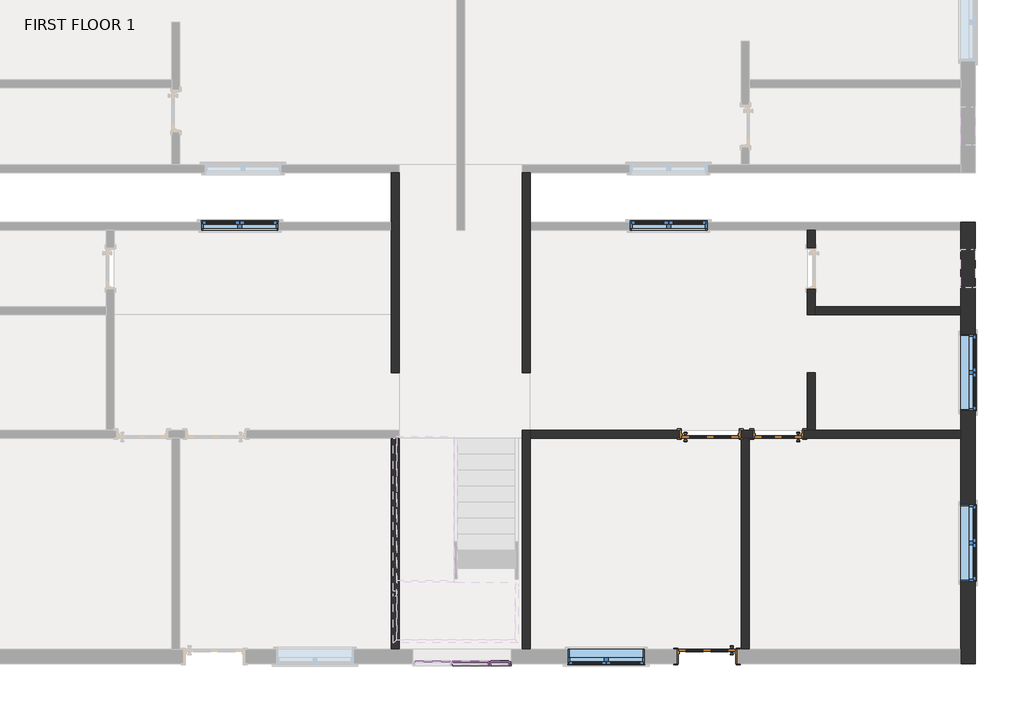
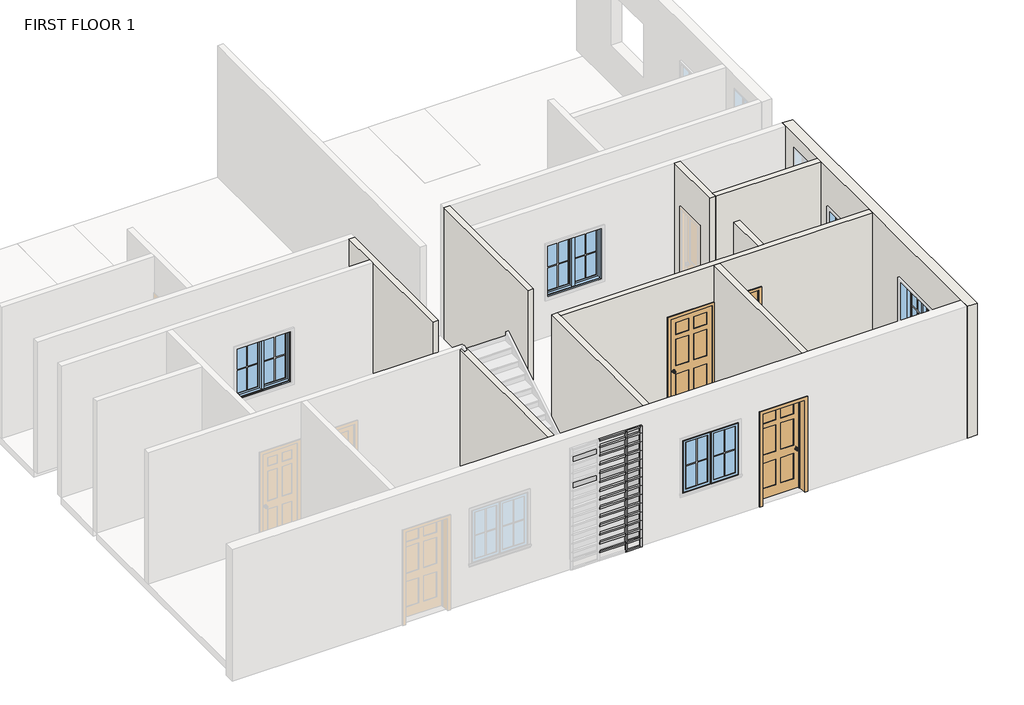
# One storey, part 2 of 4: 57 members, 18 plates, 10 walls, 5 windows, 3 doors.
"""IFC4 building model written with IfcOpenShell, lengths in millimetres."""

from ifc_helpers import new_model, si_unit, frame, origin, place, context, project, spatial, polyline, outline, extrude, faceted_brep, transform, mapped, element, save
from components import door_d66ee888, door_c610b25b, door_c5239341, member_56b223d9, member_a59c64b1, member_06854975, member_b8e7570c, member_a67f877f, member_00eacae2, member_ff422208, member_dc11c383, system_panel_glazed_b3845325, system_panel_glazed_23b8b45c, system_panel_glazed_58d257f9, system_panel_glazed_e426d894, system_panel_glazed_822b3193, window_9200f5ac, window_c2c97eee

model = new_model("IFC4")

# Units and contexts
model_context = context("Model", 3, world=origin())
ifc_project = project(units=[si_unit("LENGTHUNIT", "METRE", prefix="MILLI")], contexts=[model_context])

# Site, building, storey
site = spatial("IfcSite", under=ifc_project)
building = spatial("IfcBuilding", under=site)
storey = spatial("IfcBuildingStorey", under=building, Name="FIRST FLOOR 1", Elevation=3200.4)

# Doors
placement = place(None, origin())
door_shape = door_d66ee888(model_context)
element("IfcDoor", 1, ObjectType="Door-Interior-Single-6_Panel-Wood : 30\" x 84\"", at=placement, inside=storey, context=model_context, shape_type="MappedRepresentation", body=[
    mapped(door_shape, transform((777.5862669, -4180.7343836, 3200.4), x_axis=(-1.0, 0.0, 0.0), y_axis=(0.0, -1.0, 0.0), z_axis=(0.0, 0.0, 1.0))),
])
door_2_shape = door_c610b25b(model_context)
element("IfcDoor", 2, ObjectType="Door-Interior-Single-6_Panel-Wood : 36\" x 84\"", at=placement, inside=storey, context=model_context, shape_type="MappedRepresentation", body=[
    mapped(door_2_shape, transform((-301.9137331, -4180.7343836, 3200.4), x_axis=(1.0, 0.0, 0.0), y_axis=(0.0, 1.0, 0.0), z_axis=(0.0, 0.0, 1.0))),
])
door_3_shape = door_c5239341(model_context)
element("IfcDoor", 3, ObjectType="Door-Interior-Single-6_Panel-Wood : 36\" x 84\"", at=placement, inside=storey, context=model_context, shape_type="MappedRepresentation", body=[
    mapped(door_3_shape, transform((-352.7137331, -7704.9843836, 3200.4), x_axis=(-1.0, 0.0, 0.0), y_axis=(0.0, -1.0, 0.0), z_axis=(0.0, 0.0, 1.0))),
])

# Members
member_shape = member_56b223d9(model_context)
element("IfcMember", 4, ObjectType="Rectangular Mullion : 1.5\" x 2.5\" rectangular", at=placement, inside=storey, context=model_context, shape_type="MappedRepresentation", body=[
    mapped(member_shape, transform((-3807.0334597, -7822.4593836, 3200.4), x_axis=(1.0, 0.0, 0.0), y_axis=(0.0, -1.0, 0.0), z_axis=(0.0, 0.0, -1.0))),
])
element("IfcMember", 5, ObjectType="Rectangular Mullion : 1.5\" x 2.5\" rectangular", at=placement, inside=storey, context=model_context, shape_type="MappedRepresentation", body=[
    mapped(member_shape, transform((-3807.0334597, -7822.4593836, 3403.6), x_axis=(1.0, 0.0, 0.0), y_axis=(0.0, -1.0, 0.0), z_axis=(0.0, 0.0, -1.0))),
])
element("IfcMember", 6, ObjectType="Rectangular Mullion : 1.5\" x 2.5\" rectangular", at=placement, inside=storey, context=model_context, shape_type="MappedRepresentation", body=[
    mapped(member_shape, transform((-3807.0334597, -7822.4593836, 3606.8), x_axis=(1.0, 0.0, 0.0), y_axis=(0.0, -1.0, 0.0), z_axis=(0.0, 0.0, -1.0))),
])
element("IfcMember", 7, ObjectType="Rectangular Mullion : 1.5\" x 2.5\" rectangular", at=placement, inside=storey, context=model_context, shape_type="MappedRepresentation", body=[
    mapped(member_shape, transform((-3807.0334597, -7822.4593836, 3810.0), x_axis=(1.0, 0.0, 0.0), y_axis=(0.0, -1.0, 0.0), z_axis=(0.0, 0.0, -1.0))),
])
element("IfcMember", 8, ObjectType="Rectangular Mullion : 1.5\" x 2.5\" rectangular", at=placement, inside=storey, context=model_context, shape_type="MappedRepresentation", body=[
    mapped(member_shape, transform((-3807.0334597, -7822.4593836, 4013.2), x_axis=(1.0, 0.0, 0.0), y_axis=(0.0, -1.0, 0.0), z_axis=(0.0, 0.0, -1.0))),
])
element("IfcMember", 9, ObjectType="Rectangular Mullion : 1.5\" x 2.5\" rectangular", at=placement, inside=storey, context=model_context, shape_type="MappedRepresentation", body=[
    mapped(member_shape, transform((-3807.0334597, -7822.4593836, 4216.4), x_axis=(1.0, 0.0, 0.0), y_axis=(0.0, -1.0, 0.0), z_axis=(0.0, 0.0, -1.0))),
])
element("IfcMember", 10, ObjectType="Rectangular Mullion : 1.5\" x 2.5\" rectangular", at=placement, inside=storey, context=model_context, shape_type="MappedRepresentation", body=[
    mapped(member_shape, transform((-3807.0334597, -7822.4593836, 4419.6), x_axis=(1.0, 0.0, 0.0), y_axis=(0.0, -1.0, 0.0), z_axis=(0.0, 0.0, -1.0))),
])
element("IfcMember", 11, ObjectType="Rectangular Mullion : 1.5\" x 2.5\" rectangular", at=placement, inside=storey, context=model_context, shape_type="MappedRepresentation", body=[
    mapped(member_shape, transform((-3807.0334597, -7822.4593836, 4622.8), x_axis=(1.0, 0.0, 0.0), y_axis=(0.0, -1.0, 0.0), z_axis=(0.0, 0.0, -1.0))),
])
element("IfcMember", 12, ObjectType="Rectangular Mullion : 1.5\" x 2.5\" rectangular", at=placement, inside=storey, context=model_context, shape_type="MappedRepresentation", body=[
    mapped(member_shape, transform((-3807.0334597, -7822.4593836, 4826.0), x_axis=(1.0, 0.0, 0.0), y_axis=(0.0, -1.0, 0.0), z_axis=(0.0, 0.0, -1.0))),
])
element("IfcMember", 13, ObjectType="Rectangular Mullion : 1.5\" x 2.5\" rectangular", at=placement, inside=storey, context=model_context, shape_type="MappedRepresentation", body=[
    mapped(member_shape, transform((-3807.0334597, -7822.4593836, 5029.2), x_axis=(1.0, 0.0, 0.0), y_axis=(0.0, -1.0, 0.0), z_axis=(0.0, 0.0, -1.0))),
])
element("IfcMember", 14, ObjectType="Rectangular Mullion : 1.5\" x 2.5\" rectangular", at=placement, inside=storey, context=model_context, shape_type="MappedRepresentation", body=[
    mapped(member_shape, transform((-3807.0334597, -7822.4593836, 5232.4), x_axis=(1.0, 0.0, 0.0), y_axis=(0.0, -1.0, 0.0), z_axis=(0.0, 0.0, -1.0))),
])
element("IfcMember", 15, ObjectType="Rectangular Mullion : 1.5\" x 2.5\" rectangular", at=placement, inside=storey, context=model_context, shape_type="MappedRepresentation", body=[
    mapped(member_shape, transform((-3807.0334597, -7822.4593836, 5435.6), x_axis=(1.0, 0.0, 0.0), y_axis=(0.0, -1.0, 0.0), z_axis=(0.0, 0.0, -1.0))),
])
element("IfcMember", 16, ObjectType="Rectangular Mullion : 1.5\" x 2.5\" rectangular", at=placement, inside=storey, context=model_context, shape_type="MappedRepresentation", body=[
    mapped(member_shape, transform((-3807.0334597, -7822.4593836, 5638.8), x_axis=(1.0, 0.0, 0.0), y_axis=(0.0, -1.0, 0.0), z_axis=(0.0, 0.0, -1.0))),
])
member_2_shape = member_a59c64b1(model_context)
element("IfcMember", 17, ObjectType="Rectangular Mullion : 1.5\" x 2.5\" rectangular", at=placement, inside=storey, context=model_context, shape_type="MappedRepresentation", body=[
    mapped(member_2_shape, transform((-3807.0334597, -7822.4593836, 5842.0), x_axis=(1.0, 0.0, 0.0), y_axis=(0.0, -1.0, 0.0), z_axis=(0.0, 0.0, -1.0))),
])
member_3_shape = member_06854975(model_context)
element("IfcMember", 18, ObjectType="Rectangular Mullion : 1.5\" x 2.5\" rectangular", at=placement, inside=storey, context=model_context, shape_type="MappedRepresentation", body=[
    mapped(member_3_shape, transform((-3499.7513929, -7822.4593836, 6007.7826151), x_axis=(0.0, 0.0, 1.0), y_axis=(0.0, -1.0, 0.0), z_axis=(1.0, 0.0, 0.0))),
])
member_4_shape = member_b8e7570c(model_context)
element("IfcMember", 19, ObjectType="Rectangular Mullion : 1.5\" x 2.5\" rectangular", at=placement, inside=storey, context=model_context, shape_type="MappedRepresentation", body=[
    mapped(member_4_shape, transform((-3826.0834597, -7822.4593836, 3403.6), x_axis=(0.0, 0.0, 1.0), y_axis=(0.0, -1.0, 0.0), z_axis=(1.0, 0.0, 0.0))),
])
element("IfcMember", 20, ObjectType="Rectangular Mullion : 1.5\" x 2.5\" rectangular", at=placement, inside=storey, context=model_context, shape_type="MappedRepresentation", body=[
    mapped(member_4_shape, transform((-3826.0834597, -7822.4593836, 3606.8), x_axis=(0.0, 0.0, 1.0), y_axis=(0.0, -1.0, 0.0), z_axis=(1.0, 0.0, 0.0))),
])
element("IfcMember", 21, ObjectType="Rectangular Mullion : 1.5\" x 2.5\" rectangular", at=placement, inside=storey, context=model_context, shape_type="MappedRepresentation", body=[
    mapped(member_4_shape, transform((-3826.0834597, -7822.4593836, 3810.0), x_axis=(0.0, 0.0, 1.0), y_axis=(0.0, -1.0, 0.0), z_axis=(1.0, 0.0, 0.0))),
])
element("IfcMember", 22, ObjectType="Rectangular Mullion : 1.5\" x 2.5\" rectangular", at=placement, inside=storey, context=model_context, shape_type="MappedRepresentation", body=[
    mapped(member_4_shape, transform((-3826.0834597, -7822.4593836, 4013.2), x_axis=(0.0, 0.0, 1.0), y_axis=(0.0, -1.0, 0.0), z_axis=(1.0, 0.0, 0.0))),
])
element("IfcMember", 23, ObjectType="Rectangular Mullion : 1.5\" x 2.5\" rectangular", at=placement, inside=storey, context=model_context, shape_type="MappedRepresentation", body=[
    mapped(member_4_shape, transform((-3826.0834597, -7822.4593836, 4216.4), x_axis=(0.0, 0.0, 1.0), y_axis=(0.0, -1.0, 0.0), z_axis=(1.0, 0.0, 0.0))),
])
element("IfcMember", 24, ObjectType="Rectangular Mullion : 1.5\" x 2.5\" rectangular", at=placement, inside=storey, context=model_context, shape_type="MappedRepresentation", body=[
    mapped(member_4_shape, transform((-3826.0834597, -7822.4593836, 4419.6), x_axis=(0.0, 0.0, 1.0), y_axis=(0.0, -1.0, 0.0), z_axis=(1.0, 0.0, 0.0))),
])
element("IfcMember", 25, ObjectType="Rectangular Mullion : 1.5\" x 2.5\" rectangular", at=placement, inside=storey, context=model_context, shape_type="MappedRepresentation", body=[
    mapped(member_4_shape, transform((-3826.0834597, -7822.4593836, 4622.8), x_axis=(0.0, 0.0, 1.0), y_axis=(0.0, -1.0, 0.0), z_axis=(1.0, 0.0, 0.0))),
])
element("IfcMember", 26, ObjectType="Rectangular Mullion : 1.5\" x 2.5\" rectangular", at=placement, inside=storey, context=model_context, shape_type="MappedRepresentation", body=[
    mapped(member_4_shape, transform((-3826.0834597, -7822.4593836, 4826.0), x_axis=(0.0, 0.0, 1.0), y_axis=(0.0, -1.0, 0.0), z_axis=(1.0, 0.0, 0.0))),
])
element("IfcMember", 27, ObjectType="Rectangular Mullion : 1.5\" x 2.5\" rectangular", at=placement, inside=storey, context=model_context, shape_type="MappedRepresentation", body=[
    mapped(member_4_shape, transform((-3826.0834597, -7822.4593836, 5029.2), x_axis=(0.0, 0.0, 1.0), y_axis=(0.0, -1.0, 0.0), z_axis=(1.0, 0.0, 0.0))),
])
element("IfcMember", 28, ObjectType="Rectangular Mullion : 1.5\" x 2.5\" rectangular", at=placement, inside=storey, context=model_context, shape_type="MappedRepresentation", body=[
    mapped(member_4_shape, transform((-3826.0834597, -7822.4593836, 5232.4), x_axis=(0.0, 0.0, 1.0), y_axis=(0.0, -1.0, 0.0), z_axis=(1.0, 0.0, 0.0))),
])
element("IfcMember", 29, ObjectType="Rectangular Mullion : 1.5\" x 2.5\" rectangular", at=placement, inside=storey, context=model_context, shape_type="MappedRepresentation", body=[
    mapped(member_4_shape, transform((-3826.0834597, -7822.4593836, 5435.6), x_axis=(0.0, 0.0, 1.0), y_axis=(0.0, -1.0, 0.0), z_axis=(1.0, 0.0, 0.0))),
])
element("IfcMember", 30, ObjectType="Rectangular Mullion : 1.5\" x 2.5\" rectangular", at=placement, inside=storey, context=model_context, shape_type="MappedRepresentation", body=[
    mapped(member_4_shape, transform((-3826.0834597, -7822.4593836, 5638.8), x_axis=(0.0, 0.0, 1.0), y_axis=(0.0, -1.0, 0.0), z_axis=(1.0, 0.0, 0.0))),
])
element("IfcMember", 31, ObjectType="Rectangular Mullion : 1.5\" x 2.5\" rectangular", at=placement, inside=storey, context=model_context, shape_type="MappedRepresentation", body=[
    mapped(member_4_shape, transform((-3826.0834597, -7822.4593836, 5842.0), x_axis=(0.0, 0.0, 1.0), y_axis=(0.0, -1.0, 0.0), z_axis=(1.0, 0.0, 0.0))),
])
member_5_shape = member_a67f877f(model_context)
element("IfcMember", 32, ObjectType="Rectangular Mullion : 1.5\" x 2.5\" rectangular", at=placement, inside=storey, context=model_context, shape_type="MappedRepresentation", body=[
    mapped(member_5_shape, transform((-3826.0834597, -7822.4593836, 6007.7826151), x_axis=(0.0, 0.0, 1.0), y_axis=(0.0, -1.0, 0.0), z_axis=(1.0, 0.0, 0.0))),
])
element("IfcMember", 33, ObjectType="Rectangular Mullion : 1.5\" x 2.5\" rectangular", at=placement, inside=storey, context=model_context, shape_type="MappedRepresentation", body=[
    mapped(member_3_shape, transform((-3787.9834597, -7822.4593836, 3200.4), x_axis=(0.0, 0.0, -1.0), y_axis=(0.0, -1.0, 0.0), z_axis=(-1.0, 0.0, 0.0))),
])
member_6_shape = member_00eacae2(model_context)
element("IfcMember", 34, ObjectType="Rectangular Mullion : 1.5\" x 2.5\" rectangular", at=placement, inside=storey, context=model_context, shape_type="MappedRepresentation", body=[
    mapped(member_6_shape, transform((-3499.7513929, -7822.4593836, 3403.6), x_axis=(0.0, 0.0, 1.0), y_axis=(0.0, -1.0, 0.0), z_axis=(1.0, 0.0, 0.0))),
])
element("IfcMember", 35, ObjectType="Rectangular Mullion : 1.5\" x 2.5\" rectangular", at=placement, inside=storey, context=model_context, shape_type="MappedRepresentation", body=[
    mapped(member_6_shape, transform((-3499.7513929, -7822.4593836, 3606.8), x_axis=(0.0, 0.0, 1.0), y_axis=(0.0, -1.0, 0.0), z_axis=(1.0, 0.0, 0.0))),
])
element("IfcMember", 36, ObjectType="Rectangular Mullion : 1.5\" x 2.5\" rectangular", at=placement, inside=storey, context=model_context, shape_type="MappedRepresentation", body=[
    mapped(member_6_shape, transform((-3499.7513929, -7822.4593836, 3810.0), x_axis=(0.0, 0.0, 1.0), y_axis=(0.0, -1.0, 0.0), z_axis=(1.0, 0.0, 0.0))),
])
element("IfcMember", 37, ObjectType="Rectangular Mullion : 1.5\" x 2.5\" rectangular", at=placement, inside=storey, context=model_context, shape_type="MappedRepresentation", body=[
    mapped(member_6_shape, transform((-3499.7513929, -7822.4593836, 4013.2), x_axis=(0.0, 0.0, 1.0), y_axis=(0.0, -1.0, 0.0), z_axis=(1.0, 0.0, 0.0))),
])
element("IfcMember", 38, ObjectType="Rectangular Mullion : 1.5\" x 2.5\" rectangular", at=placement, inside=storey, context=model_context, shape_type="MappedRepresentation", body=[
    mapped(member_6_shape, transform((-3499.7513929, -7822.4593836, 4216.4), x_axis=(0.0, 0.0, 1.0), y_axis=(0.0, -1.0, 0.0), z_axis=(1.0, 0.0, 0.0))),
])
element("IfcMember", 39, ObjectType="Rectangular Mullion : 1.5\" x 2.5\" rectangular", at=placement, inside=storey, context=model_context, shape_type="MappedRepresentation", body=[
    mapped(member_6_shape, transform((-3499.7513929, -7822.4593836, 4419.6), x_axis=(0.0, 0.0, 1.0), y_axis=(0.0, -1.0, 0.0), z_axis=(1.0, 0.0, 0.0))),
])
element("IfcMember", 40, ObjectType="Rectangular Mullion : 1.5\" x 2.5\" rectangular", at=placement, inside=storey, context=model_context, shape_type="MappedRepresentation", body=[
    mapped(member_6_shape, transform((-3499.7513929, -7822.4593836, 4622.8), x_axis=(0.0, 0.0, 1.0), y_axis=(0.0, -1.0, 0.0), z_axis=(1.0, 0.0, 0.0))),
])
element("IfcMember", 41, ObjectType="Rectangular Mullion : 1.5\" x 2.5\" rectangular", at=placement, inside=storey, context=model_context, shape_type="MappedRepresentation", body=[
    mapped(member_6_shape, transform((-3499.7513929, -7822.4593836, 4826.0), x_axis=(0.0, 0.0, 1.0), y_axis=(0.0, -1.0, 0.0), z_axis=(1.0, 0.0, 0.0))),
])
element("IfcMember", 42, ObjectType="Rectangular Mullion : 1.5\" x 2.5\" rectangular", at=placement, inside=storey, context=model_context, shape_type="MappedRepresentation", body=[
    mapped(member_6_shape, transform((-3499.7513929, -7822.4593836, 5029.2), x_axis=(0.0, 0.0, 1.0), y_axis=(0.0, -1.0, 0.0), z_axis=(1.0, 0.0, 0.0))),
])
element("IfcMember", 43, ObjectType="Rectangular Mullion : 1.5\" x 2.5\" rectangular", at=placement, inside=storey, context=model_context, shape_type="MappedRepresentation", body=[
    mapped(member_6_shape, transform((-3499.7513929, -7822.4593836, 5232.4), x_axis=(0.0, 0.0, 1.0), y_axis=(0.0, -1.0, 0.0), z_axis=(1.0, 0.0, 0.0))),
])
element("IfcMember", 44, ObjectType="Rectangular Mullion : 1.5\" x 2.5\" rectangular", at=placement, inside=storey, context=model_context, shape_type="MappedRepresentation", body=[
    mapped(member_6_shape, transform((-3499.7513929, -7822.4593836, 5435.6), x_axis=(0.0, 0.0, 1.0), y_axis=(0.0, -1.0, 0.0), z_axis=(1.0, 0.0, 0.0))),
])
element("IfcMember", 45, ObjectType="Rectangular Mullion : 1.5\" x 2.5\" rectangular", at=placement, inside=storey, context=model_context, shape_type="MappedRepresentation", body=[
    mapped(member_6_shape, transform((-3499.7513929, -7822.4593836, 5638.8), x_axis=(0.0, 0.0, 1.0), y_axis=(0.0, -1.0, 0.0), z_axis=(1.0, 0.0, 0.0))),
])
element("IfcMember", 46, ObjectType="Rectangular Mullion : 1.5\" x 2.5\" rectangular", at=placement, inside=storey, context=model_context, shape_type="MappedRepresentation", body=[
    mapped(member_6_shape, transform((-3499.7513929, -7822.4593836, 5842.0), x_axis=(0.0, 0.0, 1.0), y_axis=(0.0, -1.0, 0.0), z_axis=(1.0, 0.0, 0.0))),
])
member_7_shape = member_ff422208(model_context)
element("IfcMember", 47, ObjectType="Rectangular Mullion : 1.5\" x 2.5\" rectangular", at=placement, inside=storey, context=model_context, shape_type="MappedRepresentation", body=[
    mapped(member_7_shape, transform((-3461.6513929, -7822.4593836, 3200.4), x_axis=(1.0, 0.0, 0.0), y_axis=(0.0, -1.0, 0.0), z_axis=(0.0, 0.0, -1.0))),
])
element("IfcMember", 48, ObjectType="Rectangular Mullion : 1.5\" x 2.5\" rectangular", at=placement, inside=storey, context=model_context, shape_type="MappedRepresentation", body=[
    mapped(member_7_shape, transform((-3461.6513929, -7822.4593836, 3403.6), x_axis=(1.0, 0.0, 0.0), y_axis=(0.0, -1.0, 0.0), z_axis=(0.0, 0.0, -1.0))),
])
element("IfcMember", 49, ObjectType="Rectangular Mullion : 1.5\" x 2.5\" rectangular", at=placement, inside=storey, context=model_context, shape_type="MappedRepresentation", body=[
    mapped(member_7_shape, transform((-3461.6513929, -7822.4593836, 3606.8), x_axis=(1.0, 0.0, 0.0), y_axis=(0.0, -1.0, 0.0), z_axis=(0.0, 0.0, -1.0))),
])
element("IfcMember", 50, ObjectType="Rectangular Mullion : 1.5\" x 2.5\" rectangular", at=placement, inside=storey, context=model_context, shape_type="MappedRepresentation", body=[
    mapped(member_7_shape, transform((-3461.6513929, -7822.4593836, 3810.0), x_axis=(1.0, 0.0, 0.0), y_axis=(0.0, -1.0, 0.0), z_axis=(0.0, 0.0, -1.0))),
])
element("IfcMember", 51, ObjectType="Rectangular Mullion : 1.5\" x 2.5\" rectangular", at=placement, inside=storey, context=model_context, shape_type="MappedRepresentation", body=[
    mapped(member_7_shape, transform((-3461.6513929, -7822.4593836, 4013.2), x_axis=(1.0, 0.0, 0.0), y_axis=(0.0, -1.0, 0.0), z_axis=(0.0, 0.0, -1.0))),
])
element("IfcMember", 52, ObjectType="Rectangular Mullion : 1.5\" x 2.5\" rectangular", at=placement, inside=storey, context=model_context, shape_type="MappedRepresentation", body=[
    mapped(member_7_shape, transform((-3461.6513929, -7822.4593836, 4216.4), x_axis=(1.0, 0.0, 0.0), y_axis=(0.0, -1.0, 0.0), z_axis=(0.0, 0.0, -1.0))),
])
element("IfcMember", 53, ObjectType="Rectangular Mullion : 1.5\" x 2.5\" rectangular", at=placement, inside=storey, context=model_context, shape_type="MappedRepresentation", body=[
    mapped(member_7_shape, transform((-3461.6513929, -7822.4593836, 4419.6), x_axis=(1.0, 0.0, 0.0), y_axis=(0.0, -1.0, 0.0), z_axis=(0.0, 0.0, -1.0))),
])
element("IfcMember", 54, ObjectType="Rectangular Mullion : 1.5\" x 2.5\" rectangular", at=placement, inside=storey, context=model_context, shape_type="MappedRepresentation", body=[
    mapped(member_7_shape, transform((-3461.6513929, -7822.4593836, 4622.8), x_axis=(1.0, 0.0, 0.0), y_axis=(0.0, -1.0, 0.0), z_axis=(0.0, 0.0, -1.0))),
])
element("IfcMember", 55, ObjectType="Rectangular Mullion : 1.5\" x 2.5\" rectangular", at=placement, inside=storey, context=model_context, shape_type="MappedRepresentation", body=[
    mapped(member_7_shape, transform((-3461.6513929, -7822.4593836, 4826.0), x_axis=(1.0, 0.0, 0.0), y_axis=(0.0, -1.0, 0.0), z_axis=(0.0, 0.0, -1.0))),
])
element("IfcMember", 56, ObjectType="Rectangular Mullion : 1.5\" x 2.5\" rectangular", at=placement, inside=storey, context=model_context, shape_type="MappedRepresentation", body=[
    mapped(member_7_shape, transform((-3461.6513929, -7822.4593836, 5029.2), x_axis=(1.0, 0.0, 0.0), y_axis=(0.0, -1.0, 0.0), z_axis=(0.0, 0.0, -1.0))),
])
element("IfcMember", 57, ObjectType="Rectangular Mullion : 1.5\" x 2.5\" rectangular", at=placement, inside=storey, context=model_context, shape_type="MappedRepresentation", body=[
    mapped(member_7_shape, transform((-3461.6513929, -7822.4593836, 5232.4), x_axis=(1.0, 0.0, 0.0), y_axis=(0.0, -1.0, 0.0), z_axis=(0.0, 0.0, -1.0))),
])
element("IfcMember", 58, ObjectType="Rectangular Mullion : 1.5\" x 2.5\" rectangular", at=placement, inside=storey, context=model_context, shape_type="MappedRepresentation", body=[
    mapped(member_7_shape, transform((-3461.6513929, -7822.4593836, 5435.6), x_axis=(1.0, 0.0, 0.0), y_axis=(0.0, -1.0, 0.0), z_axis=(0.0, 0.0, -1.0))),
])
element("IfcMember", 59, ObjectType="Rectangular Mullion : 1.5\" x 2.5\" rectangular", at=placement, inside=storey, context=model_context, shape_type="MappedRepresentation", body=[
    mapped(member_7_shape, transform((-3461.6513929, -7822.4593836, 5638.8), x_axis=(1.0, 0.0, 0.0), y_axis=(0.0, -1.0, 0.0), z_axis=(0.0, 0.0, -1.0))),
])
member_8_shape = member_dc11c383(model_context)
element("IfcMember", 60, ObjectType="Rectangular Mullion : 1.5\" x 2.5\" rectangular", at=placement, inside=storey, context=model_context, shape_type="MappedRepresentation", body=[
    mapped(member_8_shape, transform((-3461.6513929, -7822.4593836, 5842.0), x_axis=(1.0, 0.0, 0.0), y_axis=(0.0, -1.0, 0.0), z_axis=(0.0, 0.0, -1.0))),
])

# Plates
system_panel_glazed_shape = system_panel_glazed_b3845325(model_context)
element("IfcPlate", 61, ObjectType="System Panel : Glazed", at=placement, inside=storey, context=model_context, shape_type="MappedRepresentation", body=[
    mapped(system_panel_glazed_shape, transform((-4711.9084599, -7822.4593836, 5048.25), x_axis=(1.0, 0.0, 0.0), y_axis=(0.0, 1.0, 0.0), z_axis=(0.0, 0.0, 1.0))),
])
element("IfcPlate", 62, ObjectType="System Panel : Glazed", at=placement, inside=storey, context=model_context, shape_type="MappedRepresentation", body=[
    mapped(system_panel_glazed_shape, transform((-4711.9084599, -7822.4593836, 5657.85), x_axis=(1.0, 0.0, 0.0), y_axis=(0.0, 1.0, 0.0), z_axis=(0.0, 0.0, 1.0))),
])
system_panel_glazed_2_shape = system_panel_glazed_23b8b45c(model_context)
element("IfcPlate", 63, ObjectType="System Panel : Glazed", at=placement, inside=storey, context=model_context, shape_type="MappedRepresentation", body=[
    mapped(system_panel_glazed_2_shape, transform((-4111.8334597, -7822.4593836, 5048.25), x_axis=(1.0, 0.0, 0.0), y_axis=(0.0, 1.0, 0.0), z_axis=(0.0, 0.0, 1.0))),
])
element("IfcPlate", 64, ObjectType="System Panel : Glazed", at=placement, inside=storey, context=model_context, shape_type="MappedRepresentation", body=[
    mapped(system_panel_glazed_2_shape, transform((-4111.8334597, -7822.4593836, 5657.85), x_axis=(1.0, 0.0, 0.0), y_axis=(0.0, 1.0, 0.0), z_axis=(0.0, 0.0, 1.0))),
])
system_panel_glazed_3_shape = system_panel_glazed_58d257f9(model_context)
element("IfcPlate", 65, ObjectType="System Panel : Glazed", at=placement, inside=storey, context=model_context, shape_type="MappedRepresentation", body=[
    mapped(system_panel_glazed_3_shape, transform((-3643.8674263, -7822.4593836, 3238.5), x_axis=(1.0, 0.0, 0.0), y_axis=(0.0, 1.0, 0.0), z_axis=(0.0, 0.0, 1.0))),
])
system_panel_glazed_4_shape = system_panel_glazed_e426d894(model_context)
element("IfcPlate", 66, ObjectType="System Panel : Glazed", at=placement, inside=storey, context=model_context, shape_type="MappedRepresentation", body=[
    mapped(system_panel_glazed_4_shape, transform((-3643.8674263, -7822.4593836, 3422.65), x_axis=(1.0, 0.0, 0.0), y_axis=(0.0, 1.0, 0.0), z_axis=(0.0, 0.0, 1.0))),
])
element("IfcPlate", 67, ObjectType="System Panel : Glazed", at=placement, inside=storey, context=model_context, shape_type="MappedRepresentation", body=[
    mapped(system_panel_glazed_4_shape, transform((-3643.8674263, -7822.4593836, 3625.85), x_axis=(1.0, 0.0, 0.0), y_axis=(0.0, 1.0, 0.0), z_axis=(0.0, 0.0, 1.0))),
])
element("IfcPlate", 68, ObjectType="System Panel : Glazed", at=placement, inside=storey, context=model_context, shape_type="MappedRepresentation", body=[
    mapped(system_panel_glazed_4_shape, transform((-3643.8674263, -7822.4593836, 4032.25), x_axis=(1.0, 0.0, 0.0), y_axis=(0.0, 1.0, 0.0), z_axis=(0.0, 0.0, 1.0))),
])
element("IfcPlate", 69, ObjectType="System Panel : Glazed", at=placement, inside=storey, context=model_context, shape_type="MappedRepresentation", body=[
    mapped(system_panel_glazed_4_shape, transform((-3643.8674263, -7822.4593836, 4235.45), x_axis=(1.0, 0.0, 0.0), y_axis=(0.0, 1.0, 0.0), z_axis=(0.0, 0.0, 1.0))),
])
element("IfcPlate", 70, ObjectType="System Panel : Glazed", at=placement, inside=storey, context=model_context, shape_type="MappedRepresentation", body=[
    mapped(system_panel_glazed_4_shape, transform((-3643.8674263, -7822.4593836, 4641.85), x_axis=(1.0, 0.0, 0.0), y_axis=(0.0, 1.0, 0.0), z_axis=(0.0, 0.0, 1.0))),
])
element("IfcPlate", 71, ObjectType="System Panel : Glazed", at=placement, inside=storey, context=model_context, shape_type="MappedRepresentation", body=[
    mapped(system_panel_glazed_4_shape, transform((-3643.8674263, -7822.4593836, 4845.05), x_axis=(1.0, 0.0, 0.0), y_axis=(0.0, 1.0, 0.0), z_axis=(0.0, 0.0, 1.0))),
])
element("IfcPlate", 72, ObjectType="System Panel : Glazed", at=placement, inside=storey, context=model_context, shape_type="MappedRepresentation", body=[
    mapped(system_panel_glazed_4_shape, transform((-3643.8674263, -7822.4593836, 5251.45), x_axis=(1.0, 0.0, 0.0), y_axis=(0.0, 1.0, 0.0), z_axis=(0.0, 0.0, 1.0))),
])
element("IfcPlate", 73, ObjectType="System Panel : Glazed", at=placement, inside=storey, context=model_context, shape_type="MappedRepresentation", body=[
    mapped(system_panel_glazed_4_shape, transform((-3643.8674263, -7822.4593836, 5454.65), x_axis=(1.0, 0.0, 0.0), y_axis=(0.0, 1.0, 0.0), z_axis=(0.0, 0.0, 1.0))),
])
element("IfcPlate", 74, ObjectType="System Panel : Glazed", at=placement, inside=storey, context=model_context, shape_type="MappedRepresentation", body=[
    mapped(system_panel_glazed_4_shape, transform((-3643.8674263, -7822.4593836, 3829.05), x_axis=(1.0, 0.0, 0.0), y_axis=(0.0, 1.0, 0.0), z_axis=(0.0, 0.0, 1.0))),
])
element("IfcPlate", 75, ObjectType="System Panel : Glazed", at=placement, inside=storey, context=model_context, shape_type="MappedRepresentation", body=[
    mapped(system_panel_glazed_4_shape, transform((-3643.8674263, -7822.4593836, 4438.65), x_axis=(1.0, 0.0, 0.0), y_axis=(0.0, 1.0, 0.0), z_axis=(0.0, 0.0, 1.0))),
])
element("IfcPlate", 76, ObjectType="System Panel : Glazed", at=placement, inside=storey, context=model_context, shape_type="MappedRepresentation", body=[
    mapped(system_panel_glazed_4_shape, transform((-3643.8674263, -7822.4593836, 5048.25), x_axis=(1.0, 0.0, 0.0), y_axis=(0.0, 1.0, 0.0), z_axis=(0.0, 0.0, 1.0))),
])
element("IfcPlate", 77, ObjectType="System Panel : Glazed", at=placement, inside=storey, context=model_context, shape_type="MappedRepresentation", body=[
    mapped(system_panel_glazed_4_shape, transform((-3643.8674263, -7822.4593836, 5657.85), x_axis=(1.0, 0.0, 0.0), y_axis=(0.0, 1.0, 0.0), z_axis=(0.0, 0.0, 1.0))),
])
system_panel_glazed_5_shape = system_panel_glazed_822b3193(model_context)
element("IfcPlate", 78, ObjectType="System Panel : Glazed", at=placement, inside=storey, context=model_context, shape_type="MappedRepresentation", body=[
    mapped(system_panel_glazed_5_shape, transform((-3643.8674263, -7822.4593836, 5861.05), x_axis=(1.0, 0.0, 0.0), y_axis=(0.0, 1.0, 0.0), z_axis=(0.0, 0.0, 1.0))),
])

# Walls
element("IfcWall", 79, ObjectType="Inner Wall 5\"", at=placement, inside=storey, context=model_context, shape_type="Brep", body=[
    faceted_brep([(-5369.2137331, -24.6593836, 3200.4), (-5369.2137331, -812.0593836, 3200.4), (-5369.2137331, -939.0593836, 3200.4), (-5369.2137331, -3199.6593836, 3200.4), (-5369.2137331, -3199.6593836, 6248.4), (-5369.2137331, -939.0593836, 6248.4), (-5369.2137331, -812.0593836, 6248.4), (-5369.2137331, -24.6593836, 6248.4), (-5242.2137331, -24.6593836, 3200.4), (-5242.2137331, -24.6593836, 6248.4), (-5242.2137331, -3199.6593836, 6248.4), (-5242.2137331, -3199.6593836, 3200.4)], [[[0, 1, 2, 3, 4, 5, 6, 7]], [[8, 9, 10, 11]], [[3, 2, 1, 0, 8, 11]], [[4, 3, 11, 10]], [[7, 6, 5, 4, 10, 9]], [[0, 7, 9, 8]]]),
])
element("IfcWall", 80, ObjectType="Inner Wall 5\"", at=placement, inside=storey, context=model_context, shape_type="Brep", body=[
    faceted_brep([(-3286.4137331, -24.6593836, 3200.4), (-3286.4137331, -3199.6593836, 3200.4), (-3286.4137331, -3199.6593836, 6248.4), (-3286.4137331, -24.6593836, 6248.4), (-3159.4137331, -24.6593836, 3200.4), (-3159.4137331, -24.6593836, 6248.4), (-3159.4137331, -812.0593836, 6248.4), (-3159.4137331, -939.0593836, 6248.4), (-3159.4137331, -3199.6593836, 6248.4), (-3159.4137331, -3199.6593836, 3200.4), (-3159.4137331, -939.0593836, 3200.4), (-3159.4137331, -812.0593836, 3200.4)], [[[0, 1, 2, 3]], [[4, 5, 6, 7, 8, 9, 10, 11]], [[1, 0, 4, 11, 10, 9]], [[2, 1, 9, 8]], [[3, 2, 8, 7, 6, 5]], [[0, 3, 5, 4]]]),
])
element("IfcWall", 81, ObjectType="Inner Wall 5\"", at=placement, inside=storey, context=model_context, shape_type="Brep", body=[
    faceted_brep([(1234.7862669, -2285.2593836, 6248.4), (1234.7862669, -939.0593836, 6248.4), (1234.7862669, -939.0593836, 3200.4), (1234.7862669, -1218.4593836, 3200.4), (1234.7862669, -1218.4593836, 5359.4), (1234.7862669, -1878.8593836, 5359.4), (1234.7862669, -1878.8593836, 3200.4), (1234.7862669, -2285.2593836, 3200.4), (1361.7862669, -939.0593836, 6248.4), (1361.7862669, -2158.2593836, 6248.4), (1361.7862669, -2285.2593836, 6248.4), (1361.7862669, -2285.2593836, 3200.4), (1361.7862669, -2158.2593836, 3200.4), (1361.7862669, -1878.8593836, 3200.4), (1361.7862669, -1878.8593836, 5359.4), (1361.7862669, -1218.4593836, 5359.4), (1361.7862669, -1218.4593836, 3200.4), (1361.7862669, -939.0593836, 3200.4)], [[[0, 1, 2, 3, 4, 5, 6, 7]], [[8, 9, 10, 11, 12, 13, 14, 15, 16, 17]], [[2, 17, 16, 3]], [[11, 7, 6, 13, 12]], [[1, 0, 10, 9, 8]], [[2, 1, 8, 17]], [[0, 7, 11, 10]], [[5, 14, 13, 6]], [[14, 5, 4, 15]], [[15, 4, 3, 16]]]),
])
element("IfcWall", 82, ObjectType="Inner Wall 5\"", at=placement, inside=storey, context=model_context, shape_type="SweptSolid", body=[
    extrude(outline(polyline([(3673.1862669, -2285.2593836), (1361.7862669, -2285.2593836), (1361.7862669, -2158.2593836), (3673.1862669, -2158.2593836), (3673.1862669, -2285.2593836)])), frame((0.0, 0.0, 3200.4), z_axis=(0.0, 0.0, 1.0), x_axis=(1.0, 0.0, 0.0)), (0.0, 0.0, 1.0), 3048.0),
])
element("IfcWall", 83, ObjectType="Inner Wall 5\"", at=placement, inside=storey, context=model_context, shape_type="SweptSolid", body=[
    extrude(outline(polyline([(-5242.2137331, -4241.0593836), (-5242.2137331, -7593.8593836), (-5369.2137331, -7593.8593836), (-5369.2137331, -4241.0593836), (-5242.2137331, -4241.0593836)])), frame((0.0, 0.0, 3200.4), z_axis=(0.0, 0.0, 1.0), x_axis=(1.0, 0.0, 0.0)), (0.0, 0.0, 1.0), 3048.0),
])
element("IfcWall", 84, ObjectType="Inner Wall 5\"", at=placement, inside=storey, context=model_context, shape_type="Brep", body=[
    faceted_brep([(-3159.4137331, -7593.8593836, 3200.4), (-3159.4137331, -4241.0593836, 3200.4), (-3159.4137331, -4114.0593836, 3200.4), (-3159.4137331, -4114.0593836, 6248.4), (-3159.4137331, -4241.0593836, 6248.4), (-3159.4137331, -7593.8593836, 6248.4), (-3286.4137331, -7593.8593836, 3200.4), (-3286.4137331, -7593.8593836, 6248.4), (-3286.4137331, -4114.0593836, 6248.4), (-3286.4137331, -4114.0593836, 3200.4)], [[[0, 1, 2, 3, 4, 5]], [[6, 7, 8, 9]], [[2, 1, 0, 6, 9]], [[5, 4, 3, 8, 7]], [[0, 5, 7, 6]], [[3, 2, 9, 8]]]),
])
element("IfcWall", 85, ObjectType="Inner Wall 5\"", at=placement, inside=storey, context=model_context, shape_type="Brep", body=[
    faceted_brep([(3673.1862669, -4241.0593836, 6248.4), (320.3862669, -4241.0593836, 6248.4), (193.3862669, -4241.0593836, 6248.4), (-3159.4137331, -4241.0593836, 6248.4), (-3159.4137331, -4241.0593836, 3200.4), (-784.5137331, -4241.0593836, 3200.4), (-784.5137331, -4241.0593836, 5359.4), (180.6862669, -4241.0593836, 5359.4), (180.6862669, -4241.0593836, 3200.4), (193.3862669, -4241.0593836, 3200.4), (320.3862669, -4241.0593836, 3200.4), (371.1862669, -4241.0593836, 3200.4), (371.1862669, -4241.0593836, 5359.4), (1183.9862669, -4241.0593836, 5359.4), (1183.9862669, -4241.0593836, 3200.4), (3673.1862669, -4241.0593836, 3200.4), (-3159.4137331, -4114.0593836, 6248.4), (1234.7862669, -4114.0593836, 6248.4), (1361.7862669, -4114.0593836, 6248.4), (3673.1862669, -4114.0593836, 6248.4), (3673.1862669, -4114.0593836, 3200.4), (1361.7862669, -4114.0593836, 3200.4), (1234.7862669, -4114.0593836, 3200.4), (1183.9862669, -4114.0593836, 3200.4), (1183.9862669, -4114.0593836, 5359.4), (371.1862669, -4114.0593836, 5359.4), (371.1862669, -4114.0593836, 3200.4), (180.6862669, -4114.0593836, 3200.4), (180.6862669, -4114.0593836, 5359.4), (-784.5137331, -4114.0593836, 5359.4), (-784.5137331, -4114.0593836, 3200.4), (-3159.4137331, -4114.0593836, 3200.4)], [[[0, 1, 2, 3, 4, 5, 6, 7, 8, 9, 10, 11, 12, 13, 14, 15]], [[16, 17, 18, 19, 20, 21, 22, 23, 24, 25, 26, 27, 28, 29, 30, 31]], [[4, 31, 30, 5]], [[20, 15, 14, 23, 22, 21]], [[8, 27, 26, 11, 10, 9]], [[3, 2, 1, 0, 19, 18, 17, 16]], [[4, 3, 16, 31]], [[0, 15, 20, 19]], [[7, 28, 27, 8]], [[28, 7, 6, 29]], [[29, 6, 5, 30]], [[25, 12, 11, 26]], [[12, 25, 24, 13]], [[13, 24, 23, 14]]]),
])
element("IfcWall", 86, ObjectType="Inner Wall 5\"", at=placement, inside=storey, context=model_context, shape_type="SweptSolid", body=[
    extrude(outline(polyline([(320.3862669, -4241.0593836), (320.3862669, -7593.8593836), (193.3862669, -7593.8593836), (193.3862669, -4241.0593836), (320.3862669, -4241.0593836)])), frame((0.0, 0.0, 3200.4), z_axis=(0.0, 0.0, 1.0), x_axis=(1.0, 0.0, 0.0)), (0.0, 0.0, 1.0), 3048.0),
])
element("IfcWall", 87, ObjectType="Inner Wall 5\"", at=placement, inside=storey, context=model_context, shape_type="SweptSolid", body=[
    extrude(outline(polyline([(1361.7862669, -3199.6593836), (1361.7862669, -4114.0593836), (1234.7862669, -4114.0593836), (1234.7862669, -3199.6593836), (1361.7862669, -3199.6593836)])), frame((0.0, 0.0, 3200.4), z_axis=(0.0, 0.0, 1.0), x_axis=(1.0, 0.0, 0.0)), (0.0, 0.0, 1.0), 3048.0),
])
element("IfcWall", 88, ObjectType="outer wall 9\"", at=placement, inside=storey, context=model_context, shape_type="Brep", body=[
    faceted_brep([(3901.7862669, -7822.4593836, 3200.4), (3901.7862669, -812.0593836, 3200.4), (3901.7862669, -812.0593836, 6248.4), (3901.7862669, -7822.4593836, 6248.4), (3901.7862669, -3809.2593836, 5334.0), (3901.7862669, -2590.0593836, 5334.0), (3901.7862669, -2590.0593836, 4114.8), (3901.7862669, -3809.2593836, 4114.8), (3901.7862669, -6514.3593836, 5334.0), (3901.7862669, -5295.1593836, 5334.0), (3901.7862669, -5295.1593836, 4114.8), (3901.7862669, -6514.3593836, 4114.8), (3901.7862669, -1853.4593836, 5943.6), (3901.7862669, -1243.8593836, 5943.6), (3901.7862669, -1243.8593836, 5334.0), (3901.7862669, -1853.4593836, 5334.0), (3673.1862669, -7822.4593836, 3200.4), (3673.1862669, -7822.4593836, 6248.4), (3673.1862669, -7593.8593836, 6248.4), (3673.1862669, -4241.0593836, 6248.4), (3673.1862669, -4114.0593836, 6248.4), (3673.1862669, -2285.2593836, 6248.4), (3673.1862669, -2158.2593836, 6248.4), (3673.1862669, -939.0593836, 6248.4), (3673.1862669, -812.0593836, 6248.4), (3673.1862669, -812.0593836, 3200.4), (3673.1862669, -939.0593836, 3200.4), (3673.1862669, -2158.2593836, 3200.4), (3673.1862669, -2285.2593836, 3200.4), (3673.1862669, -4114.0593836, 3200.4), (3673.1862669, -4241.0593836, 3200.4), (3673.1862669, -7593.8593836, 3200.4), (3673.1862669, -3809.2593836, 5334.0), (3673.1862669, -3809.2593836, 4114.8), (3673.1862669, -2590.0593836, 4114.8), (3673.1862669, -2590.0593836, 5334.0), (3673.1862669, -6514.3593836, 5334.0), (3673.1862669, -6514.3593836, 4114.8), (3673.1862669, -5295.1593836, 4114.8), (3673.1862669, -5295.1593836, 5334.0), (3673.1862669, -1853.4593836, 5943.6), (3673.1862669, -1853.4593836, 5334.0), (3673.1862669, -1243.8593836, 5334.0), (3673.1862669, -1243.8593836, 5943.6)], [[[0, 1, 2, 3], [4, 5, 6, 7], [8, 9, 10, 11], [12, 13, 14, 15]], [[16, 17, 18, 19, 20, 21, 22, 23, 24, 25, 26, 27, 28, 29, 30, 31], [32, 33, 34, 35], [36, 37, 38, 39], [40, 41, 42, 43]], [[1, 0, 16, 31, 30, 29, 28, 27, 26, 25]], [[3, 2, 24, 23, 22, 21, 20, 19, 18, 17]], [[0, 3, 17, 16]], [[2, 1, 25, 24]], [[33, 32, 4, 7]], [[34, 33, 7, 6]], [[35, 34, 6, 5]], [[32, 35, 5, 4]], [[37, 36, 8, 11]], [[38, 37, 11, 10]], [[39, 38, 10, 9]], [[36, 39, 9, 8]], [[41, 40, 12, 15]], [[42, 41, 15, 14]], [[43, 42, 14, 13]], [[40, 43, 13, 12]]]),
])

# Windows
window_shape = window_9200f5ac(model_context)
element("IfcWindow", 89, ObjectType="Window-Casement-Double : 48\" x 48\"", at=placement, inside=storey, context=model_context, shape_type="MappedRepresentation", body=[
    mapped(window_shape, transform((3787.4862669, -3199.6593836, 3200.4), x_axis=(0.0, -1.0, 0.0), y_axis=(1.0, 0.0, 0.0), z_axis=(0.0, 0.0, 1.0))),
])
element("IfcWindow", 90, ObjectType="Window-Casement-Double : 48\" x 48\"", at=placement, inside=storey, context=model_context, shape_type="MappedRepresentation", body=[
    mapped(window_shape, transform((3787.4862669, -5904.7593836, 3200.4), x_axis=(0.0, -1.0, 0.0), y_axis=(1.0, 0.0, 0.0), z_axis=(0.0, 0.0, 1.0))),
])
element("IfcWindow", 91, ObjectType="Window-Casement-Double : 48\" x 48\"", at=placement, inside=storey, context=model_context, shape_type="MappedRepresentation", body=[
    mapped(window_shape, transform((-1952.9137331, -7708.1593836, 3200.4), x_axis=(-1.0, 0.0, 0.0), y_axis=(0.0, -1.0, 0.0), z_axis=(0.0, 0.0, 1.0))),
])
window_2_shape = window_c2c97eee(model_context)
element("IfcWindow", 92, ObjectType="Window-Casement-Double : 48\" x 48\"", at=placement, inside=storey, context=model_context, shape_type="MappedRepresentation", body=[
    mapped(window_2_shape, transform((-7769.5137331, -875.5593836, 3200.4), x_axis=(1.0, 0.0, 0.0), y_axis=(0.0, 1.0, 0.0), z_axis=(0.0, 0.0, 1.0))),
])
element("IfcWindow", 93, ObjectType="Window-Casement-Double : 48\" x 48\"", at=placement, inside=storey, context=model_context, shape_type="MappedRepresentation", body=[
    mapped(window_2_shape, transform((-962.3137331, -875.5593836, 3200.4), x_axis=(1.0, 0.0, 0.0), y_axis=(0.0, 1.0, 0.0), z_axis=(0.0, 0.0, 1.0))),
])

save(model, "model.ifc")

# Revit data of these elements
# Type "Door-Interior-Single-6_Panel-Wood : 30\" x 84\""
#   Type Mark = "9"
#   Assembly Code = "C1020300"
#   Analytic Construction = "Wooden"
#   Top Rail = 0' - 4 11/16"
#   Top Panel = 0' - 8"
#   Thickness = 0' - 1 3/8"
#   Thermal Resistance (R) = 2.5876 (h·ft²·°F)/BTU
#   Swing Angle [instance default] = 90.00°
#   Stiles = 0' - 4 3/4"
#   Rough Width = 2' - 8"
#   Rough Height = 7' - 1"
#   Mullion = 0' - 4 1/2"
#   Lock Rail = 0' - 7 1/2"
#   Intermediate Rail = 0' - 4 1/2"
#   Height = 7' - 0"
#   Width = 2' - 6"
#   Heat Transfer Coefficient (U) = 0.3865 BTU/(h·ft²·°F)
#   Bottom Rail = 0' - 9 1/8"
#   Trim Material = Cherry
#   Panel Material = Cherry
#   Frame Material = Cherry
#   Door Handle Material = Aluminum
#   Visual Light Transmittance = 0
#   Solar Heat Gain Coefficient = 0
#   Wall Closure = (empty or 0)
#   Function = (empty or 0)
# Type "Door-Interior-Single-6_Panel-Wood : 36\" x 84\""
#   Type Mark = "8"
#   Assembly Code = "C1020300"
#   Analytic Construction = "Wooden"
#   Top Rail = 0' - 4 11/16"
#   Top Panel = 0' - 11"
#   Thickness = 0' - 1 3/8"
#   Thermal Resistance (R) = 2.5876 (h·ft²·°F)/BTU
#   Swing Angle [instance default] = 90.00°
#   Stiles = 0' - 4 3/4"
#   Rough Width = 3' - 2"
#   Rough Height = 7' - 1"
#   Mullion = 0' - 4 1/2"
#   Lock Rail = 0' - 7 1/2"
#   Intermediate Rail = 0' - 4 1/2"
#   Height = 7' - 0"
#   Width = 3' - 0"
#   Heat Transfer Coefficient (U) = 0.3865 BTU/(h·ft²·°F)
#   Bottom Rail = 0' - 9 1/8"
#   Trim Material = Cherry
#   Panel Material = Cherry
#   Frame Material = Cherry
#   Door Handle Material = Aluminum
#   Visual Light Transmittance = 0
#   Solar Heat Gain Coefficient = 0
#   Wall Closure = (empty or 0)
#   Function = (empty or 0)
# Type "Rectangular Mullion : 1.5\" x 2.5\" rectangular"
#   built-in parameter 1007304 = 0.208333 (stored number, unit not read)
#   built-in parameter 1007301 = 0.0625 (stored number, unit not read)
#   built-in parameter 1007300 = 0.0625 (stored number, unit not read)
# Type "System Panel : Glazed"
#   Construction Type Id = "GSP4R"
#   Analytic Construction = "1/8 in Pilkington single glazing"
#   Visual Light Transmittance = 0.9
#   Solar Heat Gain Coefficient = 0.86
#   Heat Transfer Coefficient (U) = 1.18115 BTU/(h·ft²·°F)
#   Define Thermal Properties by = 1
# Type "Inner Wall 5\""
#   Assembly Code = "B2010"
#   Layers, outside or top first: 0' - 5" "wall paint" (function 1)
# Type "outer wall 9\""
#   Assembly Code = "B2010"
#   Layers, outside or top first: 0' - 9" "wall paint" (function 1)
# Type "Window-Casement-Double : 48\" x 48\""
#   Type Mark = "18"
#   Fire Rating = "0.5h"
#   Assembly Code = "B2020100"
#   Analytic Construction = "Double glazing - domestic"
#   Frame Extension [instance default] = 0' - 0 1/4"
#   Window Inset [instance default] = 0' - 0"
#   Wall Thickness [instance default] = 0' - 6"
#   Interior Wall Closure [instance default] = 0' - 2 1/4"
#   Half Width = 2' - 0"
#   Visual Light Transmittance = 0.81
#   Thermal Resistance (R) = 1.8146 (h·ft²·°F)/BTU
#   Solar Heat Gain Coefficient = 0.76
#   Rough Width = 4' - 0 1/2"
#   Rough Height = 4' - 0 1/2"
#   Height = 4' - 0"
#   Heat Transfer Coefficient (U) = 0.5511 BTU/(h·ft²·°F)
#   Exterior Wall Closure [instance default] = 0' - 1 1/4"
#   Extension Jamb [instance default] = 0' - 2 1/4"
#   Default Sill Height = 3' - 0"
#   Width = 4' - 0"
#   Muntin Visibility = yes
#   Interior Trim Visibility [instance default] = yes
#   Exterior Trim Visibility [instance default] = yes
#   Extension Jamb Visibility [instance default] = yes
#   Interior Trim Material = Wood - Stained
#   Muntin Pattern = Muntin Pattern_2x2 : Muntin Pattern_2x2
#   Interior Trim = Trim-Window-Interior-Flat : Picture Frame
#   Interior Frame Material = Wood - Stained
#   Glass Panel Material = Glass
#   Exterior Trim Material = Clad - White
#   Exterior Trim = Trim-Window-Exterior-Flat : with Sill
#   Exterior Frame Material = Clad - White
#   Wall Closure = (empty or 0)
# Element 1 (IfcDoor, "Door-Interior-Single-6_Panel-Wood : 30\" x 84\"")
#   Swing Angle = 90.00°
#   Phase Created = New Construction
#   Materials on its faces: "Cherry", "Aluminum"
# Elements 2, 3 (IfcDoor, "Door-Interior-Single-6_Panel-Wood : 36\" x 84\"")
#   Swing Angle = 90.00°
#   Phase Created = New Construction
#   Materials on its faces: "Cherry", "Aluminum"
# Elements 4, 5, 6, 7, 8, 9, 10, 11, 12, 13, 14, 15, 16, 17, 18, 19, 20, 21, 22, 23, 24, 25, 26, 27, 28, 29, 30, 31, 32, 33, 34, 35, 36, 37, 38, 39, 40, 41, 42, 43, 44, 45, 46, 47, 48, 49, 50, 51, 52, 53, 54, 55, 56, 57, 58, 59, 60 (IfcMember, "Rectangular Mullion : 1.5\" x 2.5\" rectangular")
#   Phase Created = New Construction
#   Materials on its faces: "Aluminum"
# Elements 61, 62, 63, 64, 65, 66, 67, 68, 69, 70, 71, 72, 73, 74, 75, 76, 77, 78 (IfcPlate, "System Panel : Glazed")
#   Phase Created = New Construction
#   Materials on its faces: "Glass"
# Elements 79, 80, 81, 82, 83, 84, 85, 86, 87 (IfcWall, "Inner Wall 5\"")
#   Top Offset = 0' - 0"
#   Base Offset = 0' - 0"
#   Unconnected Height = 10' - 0"
#   wall height = 10' - 0"
#   Phase Created = New Construction
#   Base Constraint = FIRST FLOOR 1
#   Materials on its faces: "wall paint"
# Element 88 (IfcWall, "outer wall 9\"")
#   Top Offset = 0' - 0"
#   Base Offset = 0' - 0"
#   Unconnected Height = 10' - 0"
#   wall height = 10' - 0"
#   Phase Created = New Construction
#   Base Constraint = FIRST FLOOR 1
#   Materials on its faces: "wall paint", "Clad - White"
# Element 89 (IfcWindow, "Window-Casement-Double : 48\" x 48\"")
#   Mark = "32"
#   Window Inset = 0' - 0"
#   Interior Wall Closure = 0' - 2 1/4"
#   Frame Extension = 0' - 0 1/4"
#   Exterior Wall Closure = 0' - 1 1/4"
#   Interior Trim Visibility = yes
#   Exterior Trim Visibility = yes
#   Phase Created = New Construction
#   Materials on its faces: "Wood - Stained", "Glass", "Clad - White"
# Element 90 (IfcWindow, "Window-Casement-Double : 48\" x 48\"")
#   Mark = "33"
#   Window Inset = 0' - 0"
#   Interior Wall Closure = 0' - 2 1/4"
#   Frame Extension = 0' - 0 1/4"
#   Exterior Wall Closure = 0' - 1 1/4"
#   Interior Trim Visibility = yes
#   Exterior Trim Visibility = yes
#   Phase Created = New Construction
#   Materials on its faces: "Wood - Stained", "Glass", "Clad - White"
# Element 91 (IfcWindow, "Window-Casement-Double : 48\" x 48\"")
#   Mark = "34"
#   Window Inset = 0' - 0"
#   Interior Wall Closure = 0' - 2 1/4"
#   Frame Extension = 0' - 0 1/4"
#   Exterior Wall Closure = 0' - 1 1/4"
#   Interior Trim Visibility = yes
#   Exterior Trim Visibility = yes
#   Phase Created = New Construction
#   Materials on its faces: "Wood - Stained", "Glass", "Clad - White"
# Element 92 (IfcWindow, "Window-Casement-Double : 48\" x 48\"")
#   Mark = "38"
#   Window Inset = 0' - 0"
#   Interior Wall Closure = 0' - 2 1/4"
#   Frame Extension = 0' - 0 1/4"
#   Exterior Wall Closure = 0' - 1 1/4"
#   Interior Trim Visibility = yes
#   Exterior Trim Visibility = yes
#   Phase Created = New Construction
#   Materials on its faces: "Wood - Stained", "Glass", "Clad - White"
# Element 93 (IfcWindow, "Window-Casement-Double : 48\" x 48\"")
#   Mark = "40"
#   Window Inset = 0' - 0"
#   Interior Wall Closure = 0' - 2 1/4"
#   Frame Extension = 0' - 0 1/4"
#   Exterior Wall Closure = 0' - 1 1/4"
#   Interior Trim Visibility = yes
#   Exterior Trim Visibility = yes
#   Phase Created = New Construction
#   Materials on its faces: "Wood - Stained", "Glass", "Clad - White"
# Materials
#   "Cherry": class "Wood", colour RGB 226 177 128, transparency 0, Description = "Prunus Serotina", Cost = 0
#   "Aluminum": class "Metal", colour RGB 247 247 247, transparency 0, Description = "Aluminum 6061", Cost = 0
#   "wall paint": class "Generic", colour RGB 120 120 120, transparency 0, Cost = 0
#   "Wood - Stained": class "Wood", colour RGB 224 178 126, transparency 0, Cost = 0
#   "Glass": class "Glass", colour RGB 0 128 192, transparency 0.75, Description = "Soda Lime Glass", Cost = 0
#   "Clad - White": class "Wood", colour RGB 242 242 238, transparency 0, Cost = 0
